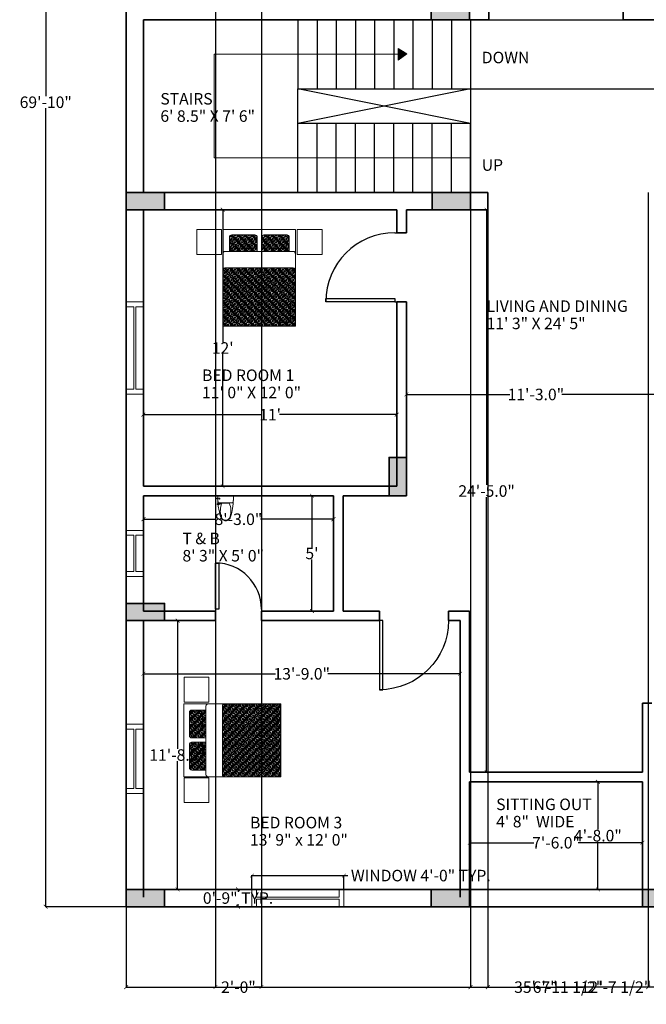
# Model space of a CAD drawing. Units: inches. Extents: x 560 to 1118, y 291 to 1226.
# Tile 1 of 4: x 560 to 886, y 291 to 804. Entities that reach past the tile are written whole.
import ezdxf

# ---------------------------------------------------------------- set-up
doc = ezdxf.new("R2010")
doc.units = ezdxf.units.IN
doc.header["$MEASUREMENT"] = 0
for name, color, linetype, lineweight in [('A-ANNO-DIMS', 2, 'Continuous', 13), ('A-ANNO-SYMB', 7, 'Continuous', 18), ('A-ANNO-TEXT', 7, 'Continuous', 18), ('A-AREA-IDEN', 7, 'Continuous', 18), ('A-COLS', 7, 'Continuous', 35), ('A-FLOR-FIXT', 9, 'Continuous', 18), ('A-FLOR-STRS', 7, 'Continuous', 25), ('DOORS', 4, 'Continuous', 25), ('FURNITURE', 8, 'Continuous', 18), ('WALL', 7, 'Continuous', 35), ('WINDOWS', 80, 'Continuous', 18)]:
    doc.layers.add(name, color=color, linetype=linetype, lineweight=lineweight)
doc.styles.get("Standard").update_dxf_attribs({"font": 'arial.ttf'})
doc.dimstyles.get("Standard").update_dxf_attribs({"dimtxt": 6, "dimasz": 2, "dimexe": 0.18, "dimexo": 0.0625, "dimgap": 0.09, "dimtad": 0, "dimtih": 1, "dimtoh": 1, "dimdec": 1, "dimzin": 0, "dimdsep": 46, "dimlunit": 3, "dimtxsty": 'Standard', "dimblk": 'ARCHTICK', "dimcen": 0.09, "dimadec": 0, "dimazin": 0, "dimtfac": 1, "dimtdec": 1, "dimtofl": 0, "dimtmove": 0, "dimatfit": 3, "dimfxl": 1, "dimtolj": 1, "dimtzin": 0, "dimarcsym": 0})
pattern_1 = [(135, (-1377.70473, -125.71507), (-0.070710678, -0.070710678), []), (135, (-1377.68705, -125.69739), (-0.070710678, -0.070710678), []), (45, (-1377.70473, -125.71507), (-0.070710678, 0.070710678), [-0.025, 0.025]), (45, (-1377.72241, -125.69739), (-0.070710678, 0.070710678), [-0.025, 0.025]), (45, (-1377.74009, -125.67972), (-0.070710678, 0.070710678), [0.025, -0.025]), (45, (-1377.75776, -125.66204), (-0.070710678, 0.070710678), [0.025, -0.025]), (135, (-1377.66938, -125.67972), (-0.070710678, -0.070710678), [0.025, -0.025]), (135, (-1377.6517, -125.66204), (-0.070710678, -0.070710678), [0.025, -0.025])]

# ---------------------------------------------------------------- blocks, each defined once
blk = doc.blocks.new('*U3')
for p, q in [((0, 0), (0, -6)), ((36, 0), (36, -6))]:
    blk.add_line(p, q)
blk.add_lwpolyline([(0, 0), (0, 36), (1.75, 36), (1.75, 0)], close=True)
blk.add_arc((0, 0), 36, 0, 90)
blk = doc.blocks.new('*U4')
for p, q in [((0, 0), (0, -6)), ((24, 0), (24, -6))]:
    blk.add_line(p, q)
blk.add_lwpolyline([(0, 0), (0, 24), (1.75, 24), (1.75, 0)], close=True)
blk.add_arc((0, 0), 24, 0, 90)
blk = doc.blocks.new('*U5')
for p, q in [((0, 0), (0, -5)), ((36, 0), (36, -5))]:
    blk.add_line(p, q)
blk.add_lwpolyline([(0, 0), (0, 36), (1.75, 36), (1.75, 0)], close=True)
blk.add_arc((0, 0), 36, 0, 90)
blk = doc.blocks.new('_ArchTick')
at = {"color": 0, "linetype": 'ByBlock', "const_width": 0.15}
blk.add_lwpolyline([(-0.5, -0.5), (0.5, 0.5)], dxfattribs=at)
blk = doc.blocks.new('*D26')
at = {"layer": 'A-ANNO-DIMS', "color": 0, "lineweight": -2, "transparency": 16777216}
for p, q in [((642.87, 491), (641.82, 491)), ((642, 491), (642, 424.15)), ((642, 351), (642, 417.85)), ((642.87, 351), (641.82, 351))]:
    blk.add_line(p, q, dxfattribs=at)
at = {"layer": 'Defpoints', "color": 0, "transparency": 16777216}
for p in [(642.93, 491), (642, 351), (642.93, 351)]:
    blk.add_point(p, dxfattribs=at)
at = {"layer": 'A-ANNO-DIMS', "color": 0, "lineweight": -2, "transparency": 16777216, "xscale": 2, "yscale": 2, "zscale": 2}
for p, rotation in [((642, 491), 90), ((642, 351), 270)]:
    blk.add_blockref('_ArchTick', p, dxfattribs=dict(at, rotation=rotation))
at = {"layer": 'A-ANNO-DIMS', "color": 0, "transparency": 16777216, "insert": (642, 421), "char_height": 6, "attachment_point": 5}
blk.add_mtext('\\A1;11\'-8.0"', dxfattribs=at)
blk = doc.blocks.new('*D27')
at = {"layer": 'A-ANNO-DIMS', "color": 0, "lineweight": -2, "transparency": 16777216}
for p, q in [((624.18, 463.36), (624.18, 463.48)), ((624.18, 463.3), (693.07, 463.3)), ((789.18, 463.3), (720.29, 463.3)), ((789.18, 463.36), (789.18, 463.48))]:
    blk.add_line(p, q, dxfattribs=at)
at = {"layer": 'Defpoints', "color": 0, "transparency": 16777216}
for p in [(624.18, 463.3), (624.18, 463.3), (789.18, 463.3)]:
    blk.add_point(p, dxfattribs=at)
at = {"layer": 'A-ANNO-DIMS', "color": 0, "lineweight": -2, "transparency": 16777216, "xscale": 2, "yscale": 2, "zscale": 2, "rotation": 180}
blk.add_blockref('_ArchTick', (624.18, 463.3), dxfattribs=at)
at = {"layer": 'A-ANNO-DIMS', "color": 0, "lineweight": -2, "transparency": 16777216, "xscale": 2, "yscale": 2, "zscale": 2}
blk.add_blockref('_ArchTick', (789.18, 463.3), dxfattribs=at)
at = {"layer": 'A-ANNO-DIMS', "color": 0, "transparency": 16777216, "insert": (706.68, 463.3), "char_height": 6, "attachment_point": 5}
blk.add_mtext('\\A1;13\'-9.0"', dxfattribs=at)
blk = doc.blocks.new('*D28')
at = {"layer": 'A-ANNO-DIMS', "color": 0, "lineweight": -2, "transparency": 16777216}
for p, q in [((712.94, 556), (711.82, 556)), ((712, 556), (712, 529.14)), ((712, 496), (712, 522.86)), ((712.94, 496), (711.82, 496))]:
    blk.add_line(p, q, dxfattribs=at)
at = {"layer": 'Defpoints', "color": 0, "transparency": 16777216}
for p in [(713, 556), (712, 496), (713, 496)]:
    blk.add_point(p, dxfattribs=at)
at = {"layer": 'A-ANNO-DIMS', "color": 0, "lineweight": -2, "transparency": 16777216, "xscale": 2, "yscale": 2, "zscale": 2}
for p, rotation in [((712, 556), 90), ((712, 496), 270)]:
    blk.add_blockref('_ArchTick', p, dxfattribs=dict(at, rotation=rotation))
at = {"layer": 'A-ANNO-DIMS', "color": 0, "transparency": 16777216, "insert": (712, 526), "char_height": 6, "attachment_point": 5}
blk.add_mtext("\\A1;5'", dxfattribs=at)
blk = doc.blocks.new('*D29')
at = {"layer": 'A-ANNO-DIMS', "color": 0, "lineweight": -2, "transparency": 16777216}
for p, q in [((624.18, 548.74), (624.18, 543.62)), ((624.18, 543.8), (662.12, 543.8)), ((723.18, 543.8), (685.24, 543.8)), ((723.18, 548.74), (723.18, 543.62))]:
    blk.add_line(p, q, dxfattribs=at)
at = {"layer": 'Defpoints', "color": 0, "transparency": 16777216}
for p in [(624.18, 548.8), (723.18, 548.8), (723.18, 543.8)]:
    blk.add_point(p, dxfattribs=at)
at = {"layer": 'A-ANNO-DIMS', "color": 0, "lineweight": -2, "transparency": 16777216, "xscale": 2, "yscale": 2, "zscale": 2, "rotation": 180}
blk.add_blockref('_ArchTick', (624.18, 543.8), dxfattribs=at)
at = {"layer": 'A-ANNO-DIMS', "color": 0, "lineweight": -2, "transparency": 16777216, "xscale": 2, "yscale": 2, "zscale": 2}
blk.add_blockref('_ArchTick', (723.18, 543.8), dxfattribs=at)
at = {"layer": 'A-ANNO-DIMS', "color": 0, "transparency": 16777216, "insert": (673.68, 543.8), "char_height": 6, "attachment_point": 5}
blk.add_mtext('\\A1;8\'-3.0"', dxfattribs=at)
blk = doc.blocks.new('*D30')
at = {"layer": 'A-ANNO-DIMS', "color": 0, "lineweight": -2, "transparency": 16777216}
for p, q in [((624.18, 598.36), (624.18, 598.48)), ((624.18, 598.3), (685.28, 598.3)), ((756.18, 598.3), (695.08, 598.3)), ((756.18, 598.36), (756.18, 598.48))]:
    blk.add_line(p, q, dxfattribs=at)
at = {"layer": 'Defpoints', "color": 0, "transparency": 16777216}
for p in [(624.18, 598.3), (756.18, 598.3), (756.18, 598.3)]:
    blk.add_point(p, dxfattribs=at)
at = {"layer": 'A-ANNO-DIMS', "color": 0, "lineweight": -2, "transparency": 16777216, "xscale": 2, "yscale": 2, "zscale": 2, "rotation": 180}
blk.add_blockref('_ArchTick', (624.18, 598.3), dxfattribs=at)
at = {"layer": 'A-ANNO-DIMS', "color": 0, "lineweight": -2, "transparency": 16777216, "xscale": 2, "yscale": 2, "zscale": 2}
blk.add_blockref('_ArchTick', (756.18, 598.3), dxfattribs=at)
at = {"layer": 'A-ANNO-DIMS', "color": 0, "transparency": 16777216, "insert": (690.18, 598.3), "char_height": 6, "attachment_point": 5}
blk.add_mtext("\\A1;11'", dxfattribs=at)
blk = doc.blocks.new('*D31')
at = {"layer": 'A-ANNO-DIMS', "color": 0, "lineweight": -2, "transparency": 16777216}
for p, q in [((663.56, 705), (665.68, 705)), ((665.5, 705), (665.5, 636.1)), ((665.5, 561), (665.5, 629.9)), ((663.56, 561), (665.68, 561))]:
    blk.add_line(p, q, dxfattribs=at)
at = {"layer": 'Defpoints', "color": 0, "transparency": 16777216}
for p in [(663.5, 705), (663.5, 561), (665.5, 561)]:
    blk.add_point(p, dxfattribs=at)
at = {"layer": 'A-ANNO-DIMS', "color": 0, "lineweight": -2, "transparency": 16777216, "xscale": 2, "yscale": 2, "zscale": 2}
for p, rotation in [((665.5, 705), 90), ((665.5, 561), 270)]:
    blk.add_blockref('_ArchTick', p, dxfattribs=dict(at, rotation=rotation))
at = {"layer": 'A-ANNO-DIMS', "color": 0, "transparency": 16777216, "insert": (665.5, 633), "char_height": 6, "attachment_point": 5}
blk.add_mtext("\\A1;12'", dxfattribs=at)
blk = doc.blocks.new('*D40')
at = {"layer": 'A-ANNO-DIMS', "color": 0, "lineweight": -2, "transparency": 16777216}
for p, q in [((794.18, 374.56), (794.18, 375.48)), ((794.18, 375.3), (827.64, 375.3)), ((884.18, 375.3), (850.72, 375.3)), ((884.18, 374.56), (884.18, 375.48))]:
    blk.add_line(p, q, dxfattribs=at)
at = {"layer": 'Defpoints', "color": 0, "transparency": 16777216}
for p in [(794.18, 374.5), (884.18, 375.3), (884.18, 374.5)]:
    blk.add_point(p, dxfattribs=at)
at = {"layer": 'A-ANNO-DIMS', "color": 0, "lineweight": -2, "transparency": 16777216, "xscale": 2, "yscale": 2, "zscale": 2, "rotation": 180}
blk.add_blockref('_ArchTick', (794.18, 375.3), dxfattribs=at)
at = {"layer": 'A-ANNO-DIMS', "color": 0, "lineweight": -2, "transparency": 16777216, "xscale": 2, "yscale": 2, "zscale": 2}
blk.add_blockref('_ArchTick', (884.18, 375.3), dxfattribs=at)
at = {"layer": 'A-ANNO-DIMS', "color": 0, "transparency": 16777216, "insert": (839.18, 375.3), "char_height": 6, "attachment_point": 5}
blk.add_mtext('\\A1;7\'-6.0"', dxfattribs=at)
blk = doc.blocks.new('*D41')
at = {"layer": 'A-ANNO-DIMS', "color": 0, "lineweight": -2, "transparency": 16777216}
for p, q in [((858.56, 407), (861.18, 407)), ((861, 407), (861, 382.15)), ((861, 351), (861, 375.85)), ((858.56, 351), (861.18, 351))]:
    blk.add_line(p, q, dxfattribs=at)
at = {"layer": 'Defpoints', "color": 0, "transparency": 16777216}
for p in [(858.5, 407), (858.5, 351), (861, 351)]:
    blk.add_point(p, dxfattribs=at)
at = {"layer": 'A-ANNO-DIMS', "color": 0, "lineweight": -2, "transparency": 16777216, "xscale": 2, "yscale": 2, "zscale": 2}
for p, rotation in [((861, 407), 90), ((861, 351), 270)]:
    blk.add_blockref('_ArchTick', p, dxfattribs=dict(at, rotation=rotation))
at = {"layer": 'A-ANNO-DIMS', "color": 0, "transparency": 16777216, "insert": (861, 379), "char_height": 6, "attachment_point": 5}
blk.add_mtext('\\A1;4\'-8.0"', dxfattribs=at)
blk = doc.blocks.new('*D42')
at = {"layer": 'A-ANNO-DIMS', "color": 0, "lineweight": -2, "transparency": 16777216}
for p, q in [((799.06, 705), (803.18, 705)), ((803, 705), (803, 561.65)), ((803, 412), (803, 555.35)), ((799.06, 412), (803.18, 412))]:
    blk.add_line(p, q, dxfattribs=at)
at = {"layer": 'Defpoints', "color": 0, "transparency": 16777216}
for p in [(799, 705), (799, 412), (803, 412)]:
    blk.add_point(p, dxfattribs=at)
at = {"layer": 'A-ANNO-DIMS', "color": 0, "lineweight": -2, "transparency": 16777216, "xscale": 2, "yscale": 2, "zscale": 2}
for p, rotation in [((803, 705), 90), ((803, 412), 270)]:
    blk.add_blockref('_ArchTick', p, dxfattribs=dict(at, rotation=rotation))
at = {"layer": 'A-ANNO-DIMS', "color": 0, "transparency": 16777216, "insert": (803, 558.5), "char_height": 6, "attachment_point": 5}
blk.add_mtext('\\A1;24\'-5.0"', dxfattribs=at)
blk = doc.blocks.new('*D43')
at = {"layer": 'A-ANNO-DIMS', "color": 0, "lineweight": -2, "transparency": 16777216}
for p, q in [((761.18, 606.56), (761.18, 608.98)), ((761.18, 608.8), (815.07, 608.8)), ((896.18, 608.8), (842.29, 608.8)), ((896.18, 606.56), (896.18, 608.98))]:
    blk.add_line(p, q, dxfattribs=at)
at = {"layer": 'Defpoints', "color": 0, "transparency": 16777216}
for p in [(761.18, 606.5), (896.18, 608.8), (896.18, 606.5)]:
    blk.add_point(p, dxfattribs=at)
at = {"layer": 'A-ANNO-DIMS', "color": 0, "lineweight": -2, "transparency": 16777216, "xscale": 2, "yscale": 2, "zscale": 2, "rotation": 180}
blk.add_blockref('_ArchTick', (761.18, 608.8), dxfattribs=at)
at = {"layer": 'A-ANNO-DIMS', "color": 0, "lineweight": -2, "transparency": 16777216, "xscale": 2, "yscale": 2, "zscale": 2}
blk.add_blockref('_ArchTick', (896.18, 608.8), dxfattribs=at)
at = {"layer": 'A-ANNO-DIMS', "color": 0, "transparency": 16777216, "insert": (828.68, 608.8), "char_height": 6, "attachment_point": 5}
blk.add_mtext('\\A1;11\'-3.0"', dxfattribs=at)
blk = doc.blocks.new('MAT-P10')
h = blk.add_hatch()
h.set_pattern_fill('BOX', color=256, scale=0.1, angle=45, style=0)
h.set_pattern_definition(pattern_1)
h.paths.add_polyline_path([(-0.157, 1.46), (0.417, 1.46), (0.417, 1.751, 0.414214), (0.367, 1.801), (-0.107, 1.801, 0.414214), (-0.157, 1.751)])
h.paths.add_polyline_path([(0.505, 1.46), (1.079, 1.46), (1.079, 1.751, 0.414214), (1.029, 1.801), (0.555, 1.801, 0.414214), (0.505, 1.751)])
h = blk.add_hatch()
h.set_pattern_fill('BOX', color=256, scale=0.1, angle=45, style=0)
h.set_pattern_definition(pattern_1)
edge = h.paths.add_edge_path()
edge.add_line((1.205, -0.085), (1.205, 1.062))
edge.add_ellipse((1.161, 1.063), major_axis=(0, 0.0568), ratio=0.776379, start_angle=270, end_angle=360)
edge.add_line((1.161, 1.119), (-0.251, 1.12))
edge.add_ellipse((-0.251, 1.063), major_axis=(0, 0.0568), ratio=0.776379, start_angle=0, end_angle=88.1396)
edge.add_line((-0.295, 1.064), (-0.295, -0.085))
edge.add_line((-0.295, -0.085), (1.205, -0.085))
for p, q in [((-0.251, 1.46), (1.161, 1.46)), ((-0.251, 1.12), (1.161, 1.119)), ((1.102, 0.406), (1.102, 0.057)), ((1.058, 0), (0.775, 0))]:
    blk.add_line(p, q)
for points in [[(-0.83, 1.909), (-0.319, 1.909), (-0.319, 1.398), (-0.83, 1.398)], [(1.205, -0.085), (-0.295, -0.085), (-0.295, 1.915), (1.205, 1.915)], [(1.244, 1.909), (1.755, 1.909), (1.755, 1.398), (1.244, 1.398)]]:
    blk.add_lwpolyline(points, close=True)
for points in [[(0.417, 1.46), (0.417, 1.751, 0.414214), (0.367, 1.801), (-0.107, 1.801, 0.414214), (-0.157, 1.751), (-0.157, 1.46)], [(1.079, 1.46), (1.079, 1.751, 0.414214), (1.029, 1.801), (0.555, 1.801, 0.414214), (0.505, 1.751), (0.505, 1.46)], [(1.012, 1.644), (1.012, 1.571, -0.414214), (0.962, 1.521), (0.753, 1.521)], [(0.37, 1.624), (0.37, 1.571, -0.414214), (0.32, 1.521), (0.111, 1.521)]]:
    blk.add_lwpolyline(points, format="xyb")
at = {"extrusion": (0, 0, -1)}
for centre, start_param, end_param in [((-0.251, 1.404), 4.712389, 6.283185), ((1.161, 1.404), 0, 1.570796), ((-0.251, 1.063), 4.712389, 6.283185), ((1.161, 1.063), 0, 1.570796), ((1.058, 0.057), 1.570796, 3.141593), ((1.058, 0.057), 1.570796, 3.141593)]:
    blk.add_ellipse(centre, major_axis=(0, 0.0568), ratio=0.776379, start_param=start_param, end_param=end_param, dxfattribs=at)
blk = doc.blocks.new('toilet-7')
at = {"color": 0, "linetype": 'ByBlock'}
for p, q in [((-0.246, -0.087), (-0.246, -0.107)), ((-0.246, -0.087), (-0.226, -0.087)), ((-0.246, -0.107), (-0.226, -0.107)), ((-0.121, -0.237), (-0.228, -0.237)), ((-0.228, -0.237), (-0.228, -0.26)), ((-0.176, -0.26), (-0.228, -0.26)), ((-0.226, -0.085), (-0.226, -0.11)), ((-0.226, -0.085), (-0.216, -0.085)), ((-0.226, -0.11), (-0.215, -0.11)), ((0.21, -0.02), (-0.21, -0.02)), ((0.199, -0.212), (-0.199, -0.212)), ((-0.18, -0.237), (-0.18, -0.212)), ((-0.176, -0.26), (-0.138, -0.245)), ((-0.138, -0.245), (-0.138, -0.237)), ((-0.121, -0.237), (-0.121, -0.212)), ((-0.102, -0.221), (0.102, -0.221)), ((0.199, -0.212), (0.21, -0.164)), ((0.215, -0.068), (0.21, -0.02)), ((0.21, -0.164), (0.215, -0.117)), ((0.215, -0.117), (0.215, -0.068))]:
    blk.add_line(p, q, dxfattribs=at)
blk.add_circle((-0.17, -0.097), 0.0125, dxfattribs=at)
for centre, radius, start, end in [((0.224, -0.092), 0.44, 170.5377, 187.7399), ((1.517, -0.087), 1.732, 181.2224, 184.9822), ((0.224, -0.092), 0.44, 187.7399, 195.822), ((1.517, -0.087), 1.732, 185.7323, 197.2477), ((0.426, -0.441), 0.572, 157.3737, 194.7786), ((-0.426, -0.441), 0.572, 345.2214, 22.6263), ((-1.517, -0.087), 1.732, 342.7523, 358.7776), ((0.012, -0.554), 0.155, 197.2477, 249.5476), ((0.022, -0.548), 0.155, 194.7786, 226.8543), ((0, -0.571), 0.122, 226.8543, 313.1457), ((0, -0.585), 0.122, 249.5476, 290.4524), ((-0.012, -0.554), 0.155, 290.4524, 342.7523), ((-0.022, -0.548), 0.155, 313.1457, 345.2214)]:
    blk.add_arc(centre, radius, start, end, dxfattribs=at)
blk = doc.blocks.new('WIN-48IN')
for p, q in [((0, 9), (48, 9)), ((0, 0), (0, 9)), ((2.5, 5), (2.5, 9)), ((45.5, 9), (45.5, 5)), ((48, 9), (48, 0)), ((48, 0), (0, 0)), ((2.5, 5), (45.5, 5)), ((2.5, 0), (2.5, 4)), ((2.5, 4), (45.5, 4)), ((45.5, 4), (45.5, 0))]:
    blk.add_line(p, q)
blk = doc.blocks.new('WIN-36IN')
for p, q in [((0, 0), (0, 36)), ((0, 36), (9, 36)), ((9, 36), (9, 0)), ((0, 33.5), (4, 33.5)), ((4, 33.5), (4, 2.5)), ((5, 33.5), (9, 33.5)), ((5, 33.5), (5, 2.5)), ((4, 2.5), (0, 2.5)), ((9, 0), (0, 0)), ((9, 2.5), (5, 2.5))]:
    blk.add_line(p, q)
blk = doc.blocks.new('WIN-24IN')
for p, q in [((0, 0), (0, 24)), ((0, 24), (9, 24)), ((0, 21.5), (4, 21.5)), ((4, 21.5), (4, 2.5)), ((5, 21.5), (9, 21.5)), ((5, 21.5), (5, 2.5)), ((9, 24), (9, 0)), ((4, 2.5), (0, 2.5)), ((9, 0), (0, 0)), ((9, 2.5), (5, 2.5))]:
    blk.add_line(p, q)
blk = doc.blocks.new('COL-RECT-9X20-NOM')
h = blk.add_hatch(color=256)
h.dxf.hatch_style = 1
h.paths.add_polyline_path([(19.98, 0), (19.98, 9), (0, 9), (0, 0)])
blk.add_lwpolyline([(0, 9), (0, 0), (19.98, 0), (19.98, 9)], close=True)
blk = doc.blocks.new('*D59')
at = {"layer": 'A-ANNO-DIMS', "color": 0, "lineweight": -2, "transparency": 16777216}
for p, q in [((680.68, 351.06), (680.68, 358.38)), ((680.68, 358.2), (728.68, 358.2)), ((728.68, 351.06), (728.68, 358.38)), ((728.68, 358.2), (730.68, 358.2))]:
    blk.add_line(p, q, dxfattribs=at)
at = {"layer": 'Defpoints', "color": 0, "transparency": 16777216}
for p in [(728.68, 358.2), (680.68, 351), (728.68, 351)]:
    blk.add_point(p, dxfattribs=at)
at = {"layer": 'A-ANNO-DIMS', "color": 0, "lineweight": -2, "transparency": 16777216, "xscale": 2, "yscale": 2, "zscale": 2, "rotation": 180}
blk.add_blockref('_ArchTick', (680.68, 358.2), dxfattribs=at)
at = {"layer": 'A-ANNO-DIMS', "color": 0, "lineweight": -2, "transparency": 16777216, "xscale": 2, "yscale": 2, "zscale": 2}
blk.add_blockref('_ArchTick', (728.68, 358.2), dxfattribs=at)
at = {"layer": 'A-ANNO-DIMS', "color": 0, "transparency": 16777216, "insert": (768.73, 358.2), "char_height": 6, "attachment_point": 5}
blk.add_mtext('\\A1;WINDOW 4\'-0" TYP.', dxfattribs=at)
blk = doc.blocks.new('*D60')
at = {"layer": 'A-ANNO-DIMS', "color": 0, "lineweight": -2, "transparency": 16777216}
for p, q in [((680.62, 351), (673.3, 351)), ((673.48, 351), (673.48, 349.65)), ((680.62, 342), (673.3, 342)), ((673.48, 342), (673.48, 343.35))]:
    blk.add_line(p, q, dxfattribs=at)
at = {"layer": 'Defpoints', "color": 0, "transparency": 16777216}
for p in [(673.48, 351), (680.68, 351), (680.68, 342)]:
    blk.add_point(p, dxfattribs=at)
at = {"layer": 'A-ANNO-DIMS', "color": 0, "lineweight": -2, "transparency": 16777216, "xscale": 2, "yscale": 2, "zscale": 2}
for p, rotation in [((673.48, 351), 90), ((673.48, 342), 270)]:
    blk.add_blockref('_ArchTick', p, dxfattribs=dict(at, rotation=rotation))
at = {"layer": 'A-ANNO-DIMS', "color": 0, "transparency": 16777216, "insert": (673.48, 346.5), "char_height": 6, "attachment_point": 5}
blk.add_mtext('\\A1;0\'-9" TYP.', dxfattribs=at)
blk = doc.blocks.new('*D71')
at = {"layer": 'A-ANNO-DIMS', "color": 0, "lineweight": -2, "transparency": 16777216}
for p, q in [((615.18, 341.94), (615.18, 299.92)), ((1042.18, 341.94), (1042.18, 299.92)), ((615.18, 300.1), (818.29, 300.1)), ((1042.18, 300.1), (839.07, 300.1))]:
    blk.add_line(p, q, dxfattribs=at)
at = {"layer": 'Defpoints', "color": 0, "transparency": 16777216}
for p in [(615.18, 342), (1042.18, 342), (1042.18, 300.1)]:
    blk.add_point(p, dxfattribs=at)
at = {"layer": 'A-ANNO-DIMS', "color": 0, "lineweight": -2, "transparency": 16777216, "xscale": 2, "yscale": 2, "zscale": 2, "rotation": 180}
blk.add_blockref('_ArchTick', (615.18, 300.1), dxfattribs=at)
at = {"layer": 'A-ANNO-DIMS', "color": 0, "lineweight": -2, "transparency": 16777216, "xscale": 2, "yscale": 2, "zscale": 2}
blk.add_blockref('_ArchTick', (1042.18, 300.1), dxfattribs=at)
at = {"layer": 'A-ANNO-DIMS', "color": 0, "transparency": 16777216, "insert": (828.68, 300.1), "char_height": 6, "attachment_point": 5}
blk.add_mtext('\\A1;35\'-7"', dxfattribs=at)
blk = doc.blocks.new('*D72')
at = {"layer": 'A-ANNO-DIMS', "color": 0, "lineweight": -2, "transparency": 16777216}
for p, q in [((615.12, 1180), (573.1, 1180)), ((573.28, 1180), (573.28, 764.15)), ((573.28, 342), (573.28, 757.85)), ((615.12, 342), (573.1, 342))]:
    blk.add_line(p, q, dxfattribs=at)
at = {"layer": 'Defpoints', "color": 0, "transparency": 16777216}
for p in [(573.28, 1180), (615.18, 1180), (615.18, 342)]:
    blk.add_point(p, dxfattribs=at)
at = {"layer": 'A-ANNO-DIMS', "color": 0, "lineweight": -2, "transparency": 16777216, "xscale": 2, "yscale": 2, "zscale": 2}
for p, rotation in [((573.28, 1180), 90), ((573.28, 342), 270)]:
    blk.add_blockref('_ArchTick', p, dxfattribs=dict(at, rotation=rotation))
at = {"layer": 'A-ANNO-DIMS', "color": 0, "transparency": 16777216, "insert": (573.28, 761), "char_height": 6, "attachment_point": 5}
blk.add_mtext('\\A1;69\'-10"', dxfattribs=at)
blk = doc.blocks.new('*D74')
at = {"layer": 'A-ANNO-DIMS', "color": 0, "lineweight": -2, "transparency": 16777216}
for p, q in [((661.68, 961.94), (661.68, 299.92)), ((685.68, 961.94), (685.68, 299.92)), ((661.68, 300.1), (665.56, 300.1)), ((685.68, 300.1), (681.8, 300.1))]:
    blk.add_line(p, q, dxfattribs=at)
at = {"layer": 'Defpoints', "color": 0, "transparency": 16777216}
for p in [(661.68, 962), (685.68, 962), (685.68, 300.1)]:
    blk.add_point(p, dxfattribs=at)
at = {"layer": 'A-ANNO-DIMS', "color": 0, "lineweight": -2, "transparency": 16777216, "xscale": 2, "yscale": 2, "zscale": 2, "rotation": 180}
blk.add_blockref('_ArchTick', (661.68, 300.1), dxfattribs=at)
at = {"layer": 'A-ANNO-DIMS', "color": 0, "lineweight": -2, "transparency": 16777216, "xscale": 2, "yscale": 2, "zscale": 2}
blk.add_blockref('_ArchTick', (685.68, 300.1), dxfattribs=at)
at = {"layer": 'A-ANNO-DIMS', "color": 0, "transparency": 16777216, "insert": (673.68, 300.1), "char_height": 6, "attachment_point": 5}
blk.add_mtext('\\A1;2\'-0"', dxfattribs=at)
blk = doc.blocks.new('*D75')
at = {"layer": 'A-ANNO-DIMS', "color": 0, "lineweight": -2, "transparency": 16777216}
for p, q in [((804.18, 804.06), (804.18, 1222.08)), ((804.18, 1221.9), (828.78, 1221.9)), ((874.18, 1221.9), (849.58, 1221.9)), ((874.18, 804.06), (874.18, 1222.08))]:
    blk.add_line(p, q, dxfattribs=at)
at = {"layer": 'Defpoints', "color": 0, "transparency": 16777216}
for p in [(874.18, 1221.9), (804.18, 804), (874.18, 804)]:
    blk.add_point(p, dxfattribs=at)
at = {"layer": 'A-ANNO-DIMS', "color": 0, "lineweight": -2, "transparency": 16777216, "xscale": 2, "yscale": 2, "zscale": 2, "rotation": 180}
blk.add_blockref('_ArchTick', (804.18, 1221.9), dxfattribs=at)
at = {"layer": 'A-ANNO-DIMS', "color": 0, "lineweight": -2, "transparency": 16777216, "xscale": 2, "yscale": 2, "zscale": 2}
blk.add_blockref('_ArchTick', (874.18, 1221.9), dxfattribs=at)
at = {"layer": 'A-ANNO-DIMS', "color": 0, "transparency": 16777216, "insert": (839.18, 1221.9), "char_height": 6, "attachment_point": 5}
blk.add_mtext('\\A1;5\'-10"', dxfattribs=at)
blk = doc.blocks.new('*D76')
at = {"layer": 'A-ANNO-DIMS', "color": 0, "lineweight": -2, "transparency": 16777216}
for p, q in [((803.64, 713.94), (803.64, 299.92)), ((887.18, 713.94), (887.18, 299.92)), ((803.64, 300.1), (828.01, 300.1)), ((887.18, 300.1), (862.81, 300.1))]:
    blk.add_line(p, q, dxfattribs=at)
at = {"layer": 'Defpoints', "color": 0, "transparency": 16777216}
for p in [(803.64, 714), (887.18, 714), (887.18, 300.1)]:
    blk.add_point(p, dxfattribs=at)
at = {"layer": 'A-ANNO-DIMS', "color": 0, "lineweight": -2, "transparency": 16777216, "xscale": 2, "yscale": 2, "zscale": 2, "rotation": 180}
blk.add_blockref('_ArchTick', (803.64, 300.1), dxfattribs=at)
at = {"layer": 'A-ANNO-DIMS', "color": 0, "lineweight": -2, "transparency": 16777216, "xscale": 2, "yscale": 2, "zscale": 2}
blk.add_blockref('_ArchTick', (887.18, 300.1), dxfattribs=at)
at = {"layer": 'A-ANNO-DIMS', "color": 0, "transparency": 16777216, "insert": (845.41, 300.1), "char_height": 6, "attachment_point": 5}
blk.add_mtext('\\A1;6\'-11 1/2"', dxfattribs=at)
blk = doc.blocks.new('*D77')
at = {"layer": 'A-ANNO-DIMS', "color": 0, "lineweight": -2, "transparency": 16777216}
for p, q in [((946.18, 770.94), (946.18, 299.92)), ((794.64, 767.94), (794.64, 299.92)), ((794.64, 300.1), (853.3, 300.1)), ((946.18, 300.1), (887.51, 300.1))]:
    blk.add_line(p, q, dxfattribs=at)
at = {"layer": 'Defpoints', "color": 0, "transparency": 16777216}
for p in [(946.18, 771), (794.64, 768), (946.18, 300.1)]:
    blk.add_point(p, dxfattribs=at)
at = {"layer": 'A-ANNO-DIMS', "color": 0, "lineweight": -2, "transparency": 16777216, "xscale": 2, "yscale": 2, "zscale": 2, "rotation": 180}
blk.add_blockref('_ArchTick', (794.64, 300.1), dxfattribs=at)
at = {"layer": 'A-ANNO-DIMS', "color": 0, "lineweight": -2, "transparency": 16777216, "xscale": 2, "yscale": 2, "zscale": 2}
blk.add_blockref('_ArchTick', (946.18, 300.1), dxfattribs=at)
at = {"layer": 'A-ANNO-DIMS', "color": 0, "transparency": 16777216, "insert": (870.41, 300.1), "char_height": 6, "attachment_point": 5}
blk.add_mtext('\\A1;12\'-7 1/2"', dxfattribs=at)
blk = doc.blocks.new('*D78')
at = {"layer": 'A-ANNO-DIMS', "color": 0, "lineweight": -2, "transparency": 16777216}
for p, q in [((794.7, 804), (1084.26, 804)), ((1084.08, 804), (1084.08, 789.16)), ((1084.08, 768), (1084.08, 782.84)), ((794.7, 768), (1084.26, 768))]:
    blk.add_line(p, q, dxfattribs=at)
at = {"layer": 'Defpoints', "color": 0, "transparency": 16777216}
for p in [(794.64, 804), (1084.08, 804), (794.64, 768)]:
    blk.add_point(p, dxfattribs=at)
at = {"layer": 'A-ANNO-DIMS', "color": 0, "lineweight": -2, "transparency": 16777216, "xscale": 2, "yscale": 2, "zscale": 2}
for p, rotation in [((1084.08, 804), 90), ((1084.08, 768), 270)]:
    blk.add_blockref('_ArchTick', p, dxfattribs=dict(at, rotation=rotation))
at = {"layer": 'A-ANNO-DIMS', "color": 0, "transparency": 16777216, "insert": (1084.08, 786), "char_height": 6, "attachment_point": 5}
blk.add_mtext('\\A1;3\'-0"', dxfattribs=at)

msp = doc.modelspace()

# ---------------------------------------------------------------- hatches: boundary and pattern name
at = {"layer": 'A-ANNO-SYMB'}
h = msp.add_hatch(color=256, dxfattribs=at)
h.dxf.hatch_style = 1
h.paths.add_polyline_path([(761.5, 786.3), (757, 789), (757, 786), (757, 783)])

# ---------------------------------------------------------------- linework, layer by layer
for p, q in [((661, 732), (661, 786)), ((661, 786), (757, 786)), ((757, 786), (757, 789)), ((761.5, 786.3), (757, 789)), ((757, 783), (761.5, 786.3)), ((757, 786), (757, 783)), ((794.64, 732), (661, 732))]:
    msp.add_line(p, q, dxfattribs=at)
at = {"layer": 'A-FLOR-STRS'}
for p, q in [((704.64, 804), (704.64, 768)), ((714.64, 804), (714.64, 768)), ((724.64, 804), (724.64, 768)), ((734.64, 804), (734.64, 768)), ((744.64, 804), (744.64, 768)), ((754.64, 804), (754.64, 768)), ((764.64, 804), (764.64, 768)), ((774.64, 804), (774.64, 768)), ((784.64, 804), (784.64, 768)), ((794.64, 804), (794.64, 768)), ((704.64, 750), (704.64, 768)), ((704.64, 768), (794.64, 768)), ((794.64, 750), (704.64, 768)), ((794.64, 768), (704.64, 750)), ((794.64, 768), (794.64, 750)), ((704.64, 714), (704.64, 750)), ((794.64, 750), (704.64, 750)), ((714.64, 714), (714.64, 750)), ((724.64, 714), (724.64, 750)), ((734.64, 714), (734.64, 750)), ((744.64, 714), (744.64, 750)), ((754.64, 714), (754.64, 750)), ((764.64, 714), (764.64, 750)), ((774.64, 714), (774.64, 750)), ((784.64, 714), (784.64, 750)), ((794.64, 714), (794.64, 750))]:
    msp.add_line(p, q, dxfattribs=at)
at = {"layer": 'WALL'}
for p, q in [((615.18, 1180), (615.18, 342)), ((804.18, 813), (804.18, 804)), ((874.18, 804), (874.18, 813)), ((624.18, 804), (624.18, 714)), ((800.18, 804), (624.18, 804)), ((804.18, 804), (800.18, 804)), ((878.18, 804), (874.18, 804)), ((946.18, 804), (878.18, 804)), ((803.64, 714), (624.18, 714)), ((803.64, 714), (803.64, 705)), ((624.18, 705), (624.18, 561)), ((756.18, 705), (624.18, 705)), ((756.18, 705), (756.18, 693)), ((761.18, 705), (761.18, 693)), ((803.64, 705), (761.18, 705)), ((761.18, 693), (756.18, 693)), ((761.18, 657), (756.18, 657)), ((756.18, 657), (756.18, 561)), ((761.18, 657), (761.18, 556)), ((756.18, 561), (624.18, 561)), ((624.18, 556), (624.18, 496)), ((723.18, 556), (624.18, 556)), ((723.18, 556), (723.18, 496)), ((728.18, 556), (728.18, 496)), ((761.18, 556), (728.18, 556)), ((624.18, 496), (661.68, 496)), ((661.68, 496), (624.18, 496)), ((661.68, 496), (661.68, 491)), ((723.18, 496), (685.68, 496)), ((685.68, 496), (685.68, 491)), ((685.68, 496), (723.18, 496)), ((747.18, 496), (728.18, 496)), ((728.18, 496), (747.18, 496)), ((747.18, 491), (747.18, 496)), ((783.18, 491), (783.18, 496)), ((783.18, 496), (794.18, 496)), ((794.18, 496), (794.18, 412)), ((624.18, 491), (624.18, 347)), ((661.68, 491), (624.18, 491)), ((661.68, 491), (624.18, 491)), ((747.18, 491), (685.68, 491)), ((747.18, 491), (685.68, 491)), ((789.18, 491), (783.18, 491)), ((789.18, 491), (789.18, 347)), ((884.18, 448), (889.18, 448)), ((884.18, 448), (884.18, 412)), ((794.18, 412), (884.18, 412)), ((794.18, 407), (884.18, 407)), ((794.18, 407), (794.18, 342)), ((884.18, 407), (884.18, 342)), ((615.18, 351), (794.18, 351)), ((794.18, 351), (884.18, 351)), ((884.18, 351), (1042.18, 351)), ((615.18, 342), (794.18, 342)), ((794.18, 342), (884.18, 342)), ((884.18, 342), (1042.18, 342))]:
    msp.add_line(p, q, dxfattribs=at)

# ---------------------------------------------------------------- block references
at = {"layer": 'A-COLS'}
for p in [(774.2, 804), (615.18, 705), (774.66, 705), (615.18, 491), (615.18, 342), (774.2, 342), (884.18, 342)]:
    msp.add_blockref('COL-RECT-9X20-NOM', p, dxfattribs=at)
at = {"layer": 'A-COLS', "rotation": 270.0000000000005}
msp.add_blockref('COL-RECT-9X20-NOM', (752.18, 575.98), dxfattribs=at)
at = {"layer": 'A-FLOR-FIXT', "xscale": 18.9039470471375, "yscale": 18.9039470471375, "zscale": 18.9039470471375}
msp.add_blockref('toilet-7', (667, 556.38), dxfattribs=at)
at = {"layer": 'DOORS', "rotation": 90}
msp.add_blockref('*U3', (755.18, 657), dxfattribs=at)
at = {"layer": 'DOORS'}
msp.add_blockref('*U4', (661.68, 497), dxfattribs=at)
at = {"layer": 'DOORS', "xscale": -1, "rotation": 180}
msp.add_blockref('*U5', (747.18, 491), dxfattribs=at)
at = {"layer": 'FURNITURE', "xscale": 25.25, "yscale": 25.25, "zscale": 25.25}
msp.add_blockref('MAT-P10', (672.96, 646.44), dxfattribs=at)
at = {"layer": 'FURNITURE', "xscale": 25.25, "yscale": 25.25, "zscale": 25.25, "rotation": 90}
msp.add_blockref('MAT-P10', (693.61, 417.15), dxfattribs=at)
at = {"layer": 'WINDOWS'}
for name, p, rotation in [('WIN-48IN', (615.18, 657), 270.0000000000002), ('WIN-36IN', (624.18, 437), 180)]:
    msp.add_blockref(name, p, dxfattribs=dict(at, rotation=rotation))
for name, p in [('WIN-24IN', (615.18, 514)), ('WIN-48IN', (680.68, 342))]:
    msp.add_blockref(name, p, dxfattribs=at)

# ---------------------------------------------------------------- texts
at = {"layer": 'A-ANNO-TEXT'}
for s, p in [('DOWN', (800.5, 781.3)), ('UP', (800.5, 725.3))]:
    msp.add_text(s, height=6, dxfattribs=at).set_placement(p)
at = {"layer": 'A-AREA-IDEN'}
for s, p in [('STAIRS', (633, 759.8)), ('6\' 8.5" X 7\' 6"', (633, 750.8)), ('LIVING AND DINING', (803, 651.8)), ('11\' 3" X 24\' 5"', (803, 642.8)), ('BED ROOM 1', (654.73, 615.8)), ('11\' 0" X 12\' 0"', (654.73, 606.8)), ('T & B', (644.5, 530.8)), ('8\' 3" X 5\' 0"', (644.5, 521.8)), ('SITTING OUT', (808, 392.3)), ('BED ROOM 3 ', (679.73, 382.8)), ('4\' 8"  WIDE', (808, 383.3)), ('13\' 9" x 12\' 0"', (679.73, 373.8))]:
    msp.add_text(s, height=6, dxfattribs=at).set_placement(p)

# ---------------------------------------------------------------- dimensions: what is measured, and where the dimension line sits
at = {"layer": 'A-ANNO-DIMS'}
for base, p1, p2, override, picture, middle in [((874.18, 1221.9), (804.18, 804), (874.18, 804), {"dimdec": 1, "dimlfac": 1, "dimrnd": 0, "dimzin": 1, "dimdsep": 46, "dimlunit": 4, "dimfrac": 2}, '*D75', (839.18, 1221.9)), ((685.68, 300.1), (661.68, 962), (685.68, 962), {"dimdec": 1, "dimlfac": 1, "dimrnd": 0, "dimzin": 1, "dimdsep": 46, "dimlunit": 4, "dimfrac": 2}, '*D74', (673.68, 300.1)), ((946.18, 300.1), (794.64, 768), (946.18, 771), {"dimdec": 1, "dimlfac": 1, "dimrnd": 0, "dimzin": 1, "dimdsep": 46, "dimlunit": 4, "dimfrac": 2}, '*D77', (870.41, 300.1)), ((887.18, 300.1), (803.64, 714), (887.18, 714), {"dimdec": 1, "dimlfac": 1, "dimrnd": 0, "dimzin": 1, "dimdsep": 46, "dimlunit": 4, "dimfrac": 2}, '*D76', (845.41, 300.1)), ((896.18, 608.8), (761.18, 606.5), (896.18, 606.5), {"dimclrd": 0, "dimclre": 0, "dimclrt": 0}, '*D43', (828.68, 608.8)), ((756.18, 598.3), (624.18, 598.3), (756.18, 598.3), {"dimclrd": 0, "dimclre": 0, "dimclrt": 0}, '*D30', (690.18, 598.3)), ((723.18, 543.8), (624.18, 548.8), (723.18, 548.8), {"dimclrd": 0, "dimclre": 0, "dimclrt": 0}, '*D29', (673.68, 543.8)), ((624.18, 463.3), (789.18, 463.3), (624.18, 463.3), {"dimclrd": 0, "dimclre": 0, "dimclrt": 0}, '*D27', (706.68, 463.3)), ((884.18, 375.3), (794.18, 374.5), (884.18, 374.5), {"dimclrd": 0, "dimclre": 0, "dimclrt": 0}, '*D40', (839.18, 375.3)), ((1042.18, 300.1), (615.18, 342), (1042.18, 342), {"dimdec": 1, "dimlfac": 1, "dimrnd": 0, "dimzin": 1, "dimdsep": 46, "dimlunit": 4, "dimfrac": 2}, '*D71', (828.68, 300.1))]:
    dim = msp.add_linear_dim(base=base, p1=p1, p2=p2, dimstyle='Standard', override=override, dxfattribs=at)
    dim.commit()
    dim.dimension.update_dxf_attribs({"geometry": picture, "text_midpoint": middle})
for base, p1, p2, override, picture, middle in [((573.28, 1180), (615.18, 342), (615.18, 1180), {"dimdec": 1, "dimlfac": 1, "dimrnd": 0, "dimzin": 1, "dimdsep": 46, "dimlunit": 4, "dimfrac": 2}, '*D72', (573.28, 761)), ((1084.08, 804), (794.64, 768), (794.64, 804), {"dimdec": 1, "dimlfac": 1, "dimrnd": 0, "dimzin": 1, "dimdsep": 46, "dimlunit": 4, "dimfrac": 2}, '*D78', (1084.08, 786)), ((665.5, 561), (663.5, 705), (663.5, 561), {"dimclrd": 0, "dimclre": 0, "dimclrt": 0}, '*D31', (665.5, 633)), ((803, 412), (799, 705), (799, 412), {"dimclrd": 0, "dimclre": 0, "dimclrt": 0}, '*D42', (803, 558.5)), ((712, 496), (713, 556), (713, 496), {"dimclrd": 0, "dimclre": 0, "dimclrt": 0}, '*D28', (712, 526)), ((642, 351), (642.93, 491), (642.93, 351), {"dimclrd": 0, "dimclre": 0, "dimclrt": 0}, '*D26', (642, 421)), ((861, 351), (858.5, 407), (858.5, 351), {"dimclrd": 0, "dimclre": 0, "dimclrt": 0}, '*D41', (861, 379))]:
    dim = msp.add_linear_dim(base=base, p1=p1, p2=p2, angle=90, dimstyle='Standard', override=override, dxfattribs=at)
    dim.commit()
    dim.dimension.update_dxf_attribs({"geometry": picture, "text_midpoint": middle})
dim = msp.add_linear_dim(base=(728.68, 358.2), p1=(680.68, 351), p2=(728.68, 351), text='WINDOW <> TYP.', dimstyle='Standard', override={"dimdec": 1, "dimlfac": 1, "dimrnd": 0, "dimzin": 1, "dimdsep": 46, "dimlunit": 4, "dimfrac": 2}, dxfattribs=at)
dim.commit()
dim.dimension.update_dxf_attribs({"geometry": '*D59', "text_midpoint": (768.73, 358.2)})
dim = msp.add_linear_dim(base=(673.48, 351), p1=(680.68, 342), p2=(680.68, 351), angle=90, text='<> TYP.', dimstyle='Standard', override={"dimdec": 1, "dimlfac": 1, "dimrnd": 0, "dimzin": 1, "dimdsep": 46, "dimlunit": 4, "dimfrac": 2}, dxfattribs=at)
dim.commit()
dim.dimension.update_dxf_attribs({"geometry": '*D60', "text_midpoint": (673.48, 346.5)})

doc.saveas('drawing.dxf')
